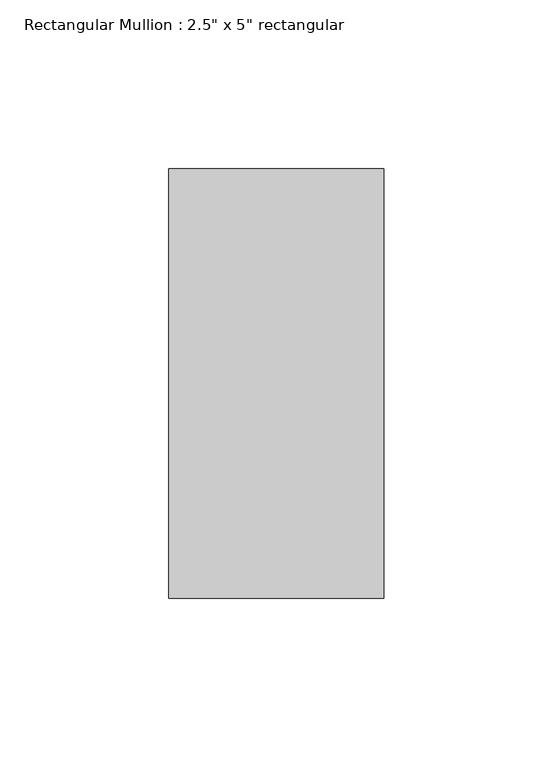
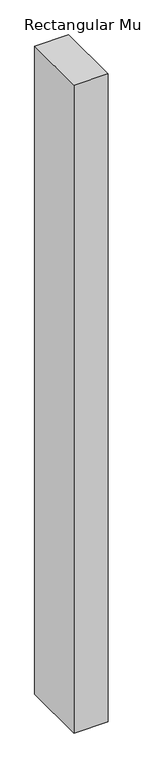
"""IFC4 building model written with IfcOpenShell, lengths in millimetres: member geometry."""

from ifc_helpers import new_model, si_unit, frame, origin, place, context, project, spatial, polyline, outline, extrude, source, transform, mapped, element, save


def member_cba00588(model_context):
    return source(origin(), model_context, "Body", "SweptSolid", [
        extrude(outline(polyline([(0.0, 63.5), (0.0, -63.5), (-63.5, -63.5), (-63.5, 63.5), (0.0, 63.5)])), frame((0.0, 0.0, -1276.35), z_axis=(0.0, 0.0, 1.0), x_axis=(1.0, 0.0, 0.0)), (0.0, 0.0, 1.0), 1276.35),
    ])


if __name__ == "__main__":
    model = new_model("IFC4")
    model_context = context("Model", 3, world=origin())
    ifc_project = project(units=[si_unit("LENGTHUNIT", "METRE", prefix="MILLI")], contexts=[model_context])
    site = spatial("IfcSite", under=ifc_project)
    building = spatial("IfcBuilding", under=site)
    placement = place(None, origin())
    member_shape = member_cba00588(model_context)
    element("IfcMember", 1, ObjectType="Rectangular Mullion : 2.5\" x 5\" rectangular", at=placement, inside=building, context=model_context, shape_type="MappedRepresentation", body=[
        mapped(member_shape, transform((0.0, 0.0, 0.0), x_axis=(1.0, 0.0, 0.0), y_axis=(0.0, 1.0, 0.0), z_axis=(0.0, 0.0, 1.0))),
    ])
    save(model, "model.ifc")

# Revit data of these elements
# Type "Rectangular Mullion : 2.5\" x 5\" rectangular"
#   built-in parameter 1007304 = 0.416667 (stored number, unit not read)
#   built-in parameter 1007301 = 0.104167 (stored number, unit not read)
#   built-in parameter 1007300 = 0.104167 (stored number, unit not read)
# Element 1 (IfcMember, "Rectangular Mullion : 2.5\" x 5\" rectangular")
#   Materials on its faces: "Iron, Ductile"
# Materials
#   "Iron, Ductile": class "Metal", colour RGB 0 0 0, transparency 0, Description = "Ductile cast iron", Cost = 0
